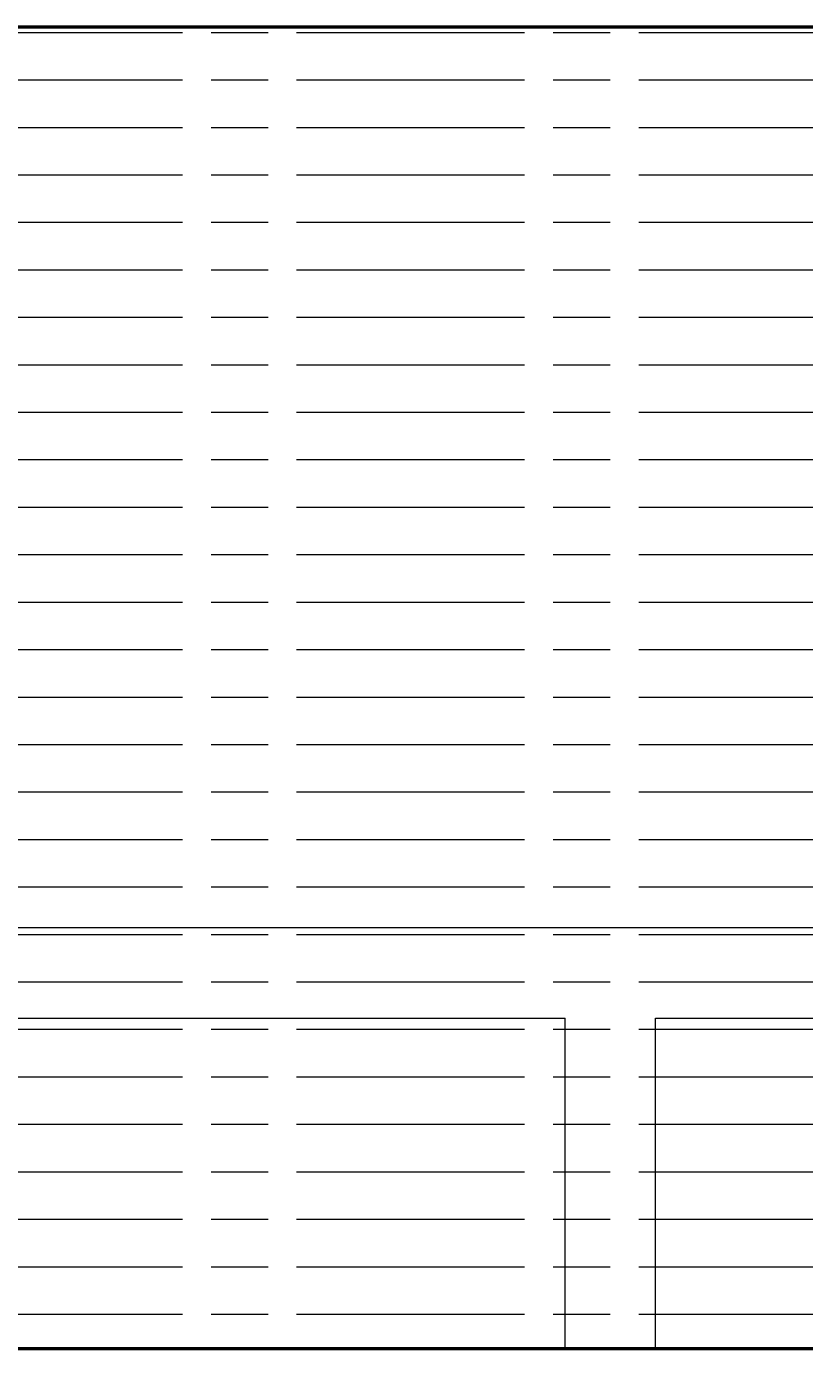
# Model space of a CAD drawing. Units: inches. Extents: x 5375 to 6084, y 16106 to 17259.
# Tile 5 of 32: x 5624 to 5705, y 16219 to 16361. Entities that reach past the tile are written whole.
import ezdxf

# ---------------------------------------------------------------- set-up
doc = ezdxf.new("R2010")
doc.units = ezdxf.units.IN
for name, color, linetype, lineweight in [('A-ANNO-DIMS', 2, 'Continuous', 18), ('C-PVMT-PATT', 2, 'Continuous', 13), ('WALL', 6, 'Continuous', 50)]:
    doc.layers.add(name, color=color, linetype=linetype, lineweight=lineweight)
doc.styles.get("Standard").update_dxf_attribs({"font": 'arial.ttf'})
doc.dimstyles.get("Standard").update_dxf_attribs({"dimtxt": 0.18, "dimasz": 0.18, "dimexe": 0.18, "dimexo": 0.0625, "dimgap": 0.09, "dimtad": 0, "dimtih": 1, "dimtoh": 1, "dimdec": 4, "dimzin": 0, "dimdsep": 46, "dimtxsty": 'Standard', "dimcen": 0.09, "dimadec": 0, "dimazin": 0, "dimtfac": 1, "dimtdec": 4, "dimtofl": 0, "dimtmove": 0, "dimatfit": 3, "dimfxl": 1, "dimtolj": 1, "dimtzin": 0, "dimarcsym": 0})

# ---------------------------------------------------------------- blocks, each defined once
blk = doc.blocks.new('*D51')
at = {"layer": 'A-ANNO-DIMS', "color": 0, "lineweight": -2, "transparency": 16777216}
for p, q in [((5820.47, 16344.39), (5761.62, 16271.02)), ((5820.65, 16344.39), (5820.47, 16344.39)), ((5663.14, 16148.34), (5663.32, 16148.34)), ((5663.23, 16148.25), (5663.23, 16148.43))]:
    blk.add_line(p, q, dxfattribs=at)
at = {"layer": 'A-ANNO-DIMS', "color": 0, "transparency": 16777216}
blk.add_solid([(5761.59, 16271.03), (5761.64, 16271), (5761.5, 16270.88)], dxfattribs=at)
at = {"layer": 'Defpoints', "color": 0, "transparency": 16777216}
for p in [(5761.5, 16270.88), (5663.23, 16148.34)]:
    blk.add_point(p, dxfattribs=at)
at = {"layer": 'A-ANNO-DIMS', "color": 0, "transparency": 16777216, "insert": (5821.2, 16344.39), "char_height": 0.18, "attachment_point": 5}
blk.add_mtext('\\A1;R157.07', dxfattribs=at)

msp = doc.modelspace()

# ---------------------------------------------------------------- hatches: boundary and pattern name
at = {"layer": 'C-PVMT-PATT'}
h = msp.add_hatch(dxfattribs=at)
h.set_pattern_fill('AR-B816C', color=256)
h.paths.add_polyline_path([(5707.6199, 16360.5793), (5479.6199, 16360.5793), (5479.6199, 16221.3785), (5802.2897, 16221.3785, 0.20288708), (5707.6199, 16299.0135)])
h = msp.add_hatch(dxfattribs=at)
h.set_pattern_fill('ACAD_ISO08W100', color=256)
h.paths.add_polyline_path([(5707.6199, 16360.5793), (5479.6199, 16360.5793), (5479.6199, 16221.3785), (5802.2897, 16221.3785, 0.20288708), (5707.6199, 16299.0135)])

# ---------------------------------------------------------------- linework, layer by layer
at = {"layer": 'WALL'}
for p, q in [((5470.6199, 16360.5793), (5707.6199, 16360.5793)), ((5479.6199, 16221.3785), (6022.6199, 16221.3785))]:
    msp.add_line(p, q, dxfattribs=at)

# ---------------------------------------------------------------- dimensions: what is measured, and where the dimension line sits
at = {"layer": 'A-ANNO-DIMS'}
dim = msp.add_radius_dim(center=(5663.2298, 16148.3446), mpoint=(5761.504, 16270.8753), dimstyle='Standard', override={"dimdec": 2, "dimlfac": 1, "dimrnd": 0, "dimzin": 0, "dimdsep": 46, "dimlunit": 2}, dxfattribs=at)
dim.commit()
dim.dimension.update_dxf_attribs({"geometry": '*D51', "text_midpoint": (5821.1984, 16344.3937), "dimtype": 164})

doc.saveas('drawing.dxf')
